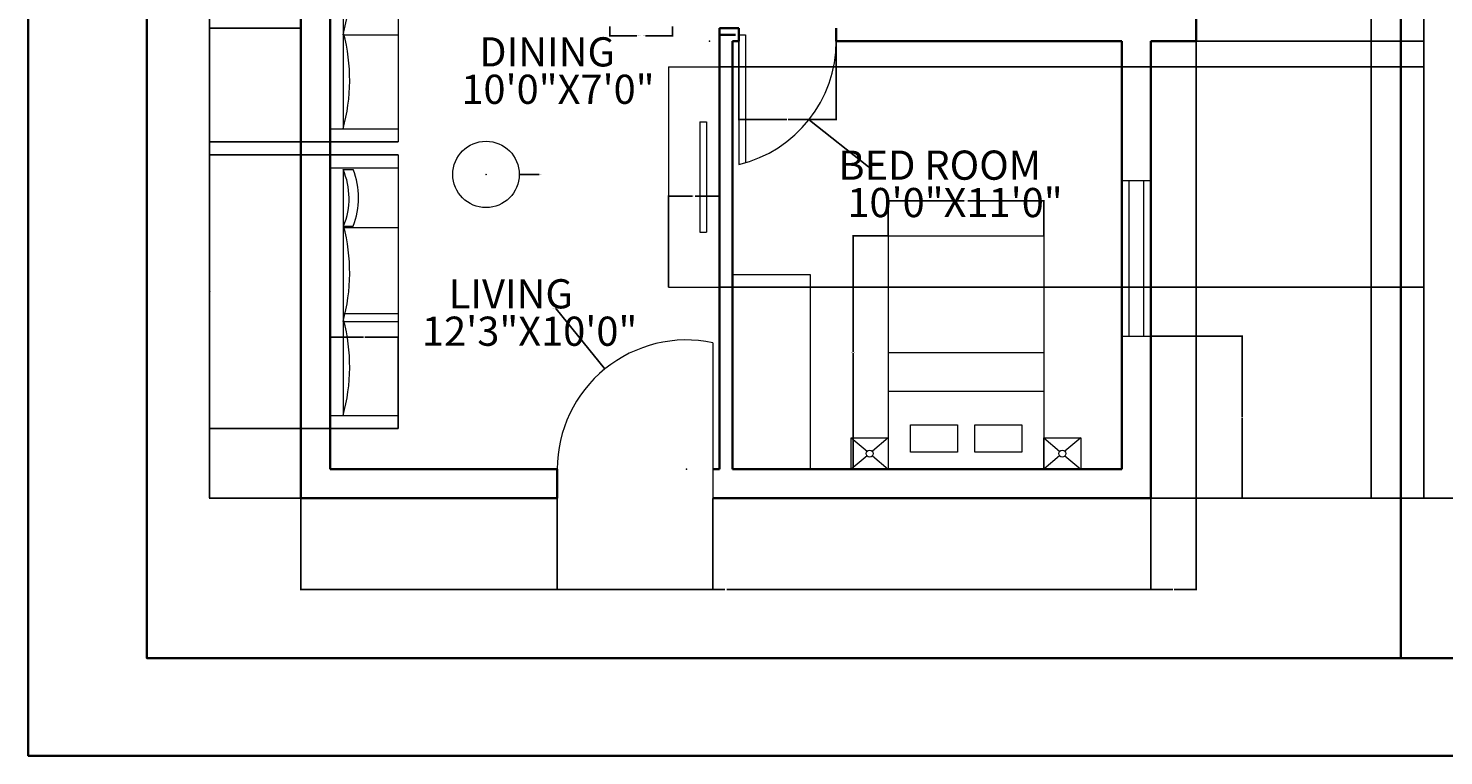
# Model space of a CAD drawing. Units: inches. Extents: x 1762 to 3150, y 1680 to 2382.
# Tile 1 of 6: x 1762 to 2199, y 1680 to 1904. Entities that reach past the tile are written whole.
import ezdxf

# ---------------------------------------------------------------- set-up
doc = ezdxf.new("R2010")
doc.units = ezdxf.units.IN
for name, color, linetype, lineweight in [('A-ANNO-DIMS', 2, 'Continuous', 18), ('A-ANNO-TTLB', 7, 'Continuous', 35), ('A-AREA-IDEN', 7, 'Continuous', 18), ('A-DOOR', 3, 'Continuous', 18), ('A-EQPM', 8, 'Continuous', 18), ('A-GLAZ', 4, 'Continuous', 18), ('A-WALL', 7, 'Continuous', 35)]:
    doc.layers.add(name, color=color, linetype=linetype, lineweight=lineweight)
doc.layers.add('A-FLOR-CASE', color=242, linetype='Continuous', lineweight=18, true_color=0xcd2027)
doc.layers.add('A-FURN', color=51, linetype='Continuous', lineweight=18, true_color=0xf7f281)
doc.styles.get("Standard").update_dxf_attribs({"font": 'arial.ttf'})
doc.dimstyles.get("Standard").update_dxf_attribs({"dimtxt": 0.18, "dimasz": 0.18, "dimexe": 0.18, "dimexo": 0.0625, "dimgap": 0.09, "dimtad": 0, "dimtih": 1, "dimtoh": 1, "dimdec": 4, "dimzin": 0, "dimdsep": 46, "dimtxsty": 'Standard', "dimcen": 0.09, "dimadec": 0, "dimazin": 0, "dimtfac": 1, "dimtdec": 4, "dimtofl": 0, "dimtmove": 0, "dimatfit": 3, "dimfxl": 1, "dimtolj": 1, "dimtzin": 0, "dimarcsym": 0})

# ---------------------------------------------------------------- blocks, each defined once
blk = doc.blocks.new('WINDOW-48IN')
for p, q in [((0, 48), (9, 48)), ((2.25, 48), (2.25, 0)), ((6.75, 48), (6.75, 0)), ((0, 0), (9, 0))]:
    blk.add_line(p, q)
blk = doc.blocks.new('BED-48X72IN')
for p, q in [((0, 72), (48, 72)), ((0, 72), (0, 0)), ((48, 72), (48, 0)), ((0, 36), (48, 36)), ((0, 24), (48, 24))]:
    blk.add_line(p, q)
for points in [[(6.88, 13.68), (21.36, 13.68), (21.36, 5.23), (6.88, 5.23)], [(26.73, 13.68), (41.21, 13.68), (41.21, 5.23), (26.73, 5.23)]]:
    blk.add_lwpolyline(points, close=True)
blk = doc.blocks.new('NIGHTSTAND')
for p, q in [((0, 9.61), (4.85, 5.5)), ((11.36, 9.61), (6.51, 5.5)), ((4.85, 4.1), (0, 0)), ((6.51, 4.1), (11.36, 0))]:
    blk.add_line(p, q)
blk.add_lwpolyline([(0, 9.61), (11.36, 9.61), (11.36, 0), (0, 0)], close=True)
blk.add_circle((5.68, 4.8), 1.08)
blk = doc.blocks.new('*D12')
at = {"layer": 'A-ANNO-DIMS', "color": 0, "lineweight": -2, "transparency": 16777216}
for p, q in [((2027.48, 1839.99), (2016.56, 1839.99)), ((2016.74, 1839.81), (2016.74, 1804.17)), ((2016.74, 1768.17), (2016.74, 1803.81)), ((2027.48, 1767.99), (2016.56, 1767.99))]:
    blk.add_line(p, q, dxfattribs=at)
at = {"layer": 'A-ANNO-DIMS', "color": 0, "transparency": 16777216}
for points in [[(2016.71, 1839.81), (2016.77, 1839.81), (2016.74, 1839.99)], [(2016.71, 1768.17), (2016.77, 1768.17), (2016.74, 1767.99)]]:
    blk.add_solid(points, dxfattribs=at)
at = {"layer": 'Defpoints', "color": 0, "transparency": 16777216}
for p in [(2016.74, 1839.99), (2027.54, 1839.99), (2027.54, 1767.99)]:
    blk.add_point(p, dxfattribs=at)
at = {"layer": 'A-ANNO-DIMS', "color": 0, "transparency": 16777216, "insert": (2016.74, 1803.99), "char_height": 0.18, "attachment_point": 5}
blk.add_mtext('\\A1;BED 72 TYP.', dxfattribs=at)
blk = doc.blocks.new('*D13')
at = {"layer": 'A-ANNO-DIMS', "color": 0, "lineweight": -2, "transparency": 16777216}
for p, q in [((2027.54, 1840.05), (2027.54, 1850.97)), ((2027.72, 1850.79), (2051.01, 1850.79)), ((2075.36, 1850.79), (2052.07, 1850.79)), ((2075.54, 1840.05), (2075.54, 1850.97))]:
    blk.add_line(p, q, dxfattribs=at)
at = {"layer": 'A-ANNO-DIMS', "color": 0, "transparency": 16777216}
for points in [[(2027.72, 1850.82), (2027.72, 1850.76), (2027.54, 1850.79)], [(2075.36, 1850.82), (2075.36, 1850.76), (2075.54, 1850.79)]]:
    blk.add_solid(points, dxfattribs=at)
at = {"layer": 'Defpoints', "color": 0, "transparency": 16777216}
for p in [(2075.54, 1850.79), (2027.54, 1839.99), (2075.54, 1839.99)]:
    blk.add_point(p, dxfattribs=at)
at = {"layer": 'A-ANNO-DIMS', "color": 0, "transparency": 16777216, "insert": (2051.54, 1850.79), "char_height": 0.18, "attachment_point": 5}
blk.add_mtext('\\A1;48 TYP.', dxfattribs=at)
blk = doc.blocks.new('*D22')
at = {"layer": 'A-ANNO-DIMS', "color": 0, "lineweight": -2, "transparency": 16777216}
for p, q in [((1941.79, 1904.51), (1941.79, 1901.5)), ((1961.03, 1904.51), (1961.03, 1901.5)), ((1941.97, 1901.68), (1950.09, 1901.68)), ((1960.85, 1901.68), (1952.73, 1901.68))]:
    blk.add_line(p, q, dxfattribs=at)
at = {"layer": 'A-ANNO-DIMS', "color": 0, "transparency": 16777216}
for points in [[(1941.97, 1901.71), (1941.97, 1901.65), (1941.79, 1901.68)], [(1960.85, 1901.71), (1960.85, 1901.65), (1961.03, 1901.68)]]:
    blk.add_solid(points, dxfattribs=at)
at = {"layer": 'Defpoints', "color": 0, "transparency": 16777216}
for p in [(1941.79, 1904.57), (1961.03, 1904.57), (1941.79, 1901.68)]:
    blk.add_point(p, dxfattribs=at)
at = {"layer": 'A-ANNO-DIMS', "color": 0, "transparency": 16777216, "insert": (1951.41, 1901.68), "char_height": 0.18, "attachment_point": 5}
blk.add_mtext('\\A1;WIDE CHAIR 19 TYP.', dxfattribs=at)
blk = doc.blocks.new('*D33')
at = {"layer": 'A-ANNO-DIMS', "color": 0, "lineweight": -2, "transparency": 16777216}
for p, q in [((1969.475966, 2232.98945), (1818.208466, 2232.98945)), ((1818.388466, 2232.80945), (1818.388466, 1996.16945)), ((1818.388466, 1759.16945), (1818.388466, 1995.80945)), ((1846.475966, 1758.98945), (1818.208466, 1758.98945))]:
    blk.add_line(p, q, dxfattribs=at)
at = {"layer": 'A-ANNO-DIMS', "color": 0, "transparency": 16777216}
for points in [[(1818.358466, 2232.80945), (1818.418466, 2232.80945), (1818.388466, 2232.98945)], [(1818.358466, 1759.16945), (1818.418466, 1759.16945), (1818.388466, 1758.98945)]]:
    blk.add_solid(points, dxfattribs=at)
at = {"layer": 'Defpoints', "color": 0, "transparency": 16777216}
for p in [(1818.388466, 2232.98945), (1969.538466, 2232.98945), (1846.538466, 1758.98945)]:
    blk.add_point(p, dxfattribs=at)
at = {"layer": 'A-ANNO-DIMS', "color": 0, "transparency": 16777216, "insert": (1818.388466, 1995.98945), "char_height": 0.18, "attachment_point": 5}
blk.add_mtext('\\A1;474', dxfattribs=at)
blk = doc.blocks.new('*D35')
at = {"layer": 'A-ANNO-DIMS', "color": 0, "lineweight": -2, "transparency": 16777216}
for p, q in [((2108.6, 1899.99), (2192.87, 1899.99)), ((2192.69, 1899.81), (2192.69, 1829.67)), ((2192.69, 1759.17), (2192.69, 1829.31)), ((2108.6, 1758.99), (2192.87, 1758.99))]:
    blk.add_line(p, q, dxfattribs=at)
at = {"layer": 'A-ANNO-DIMS', "color": 0, "transparency": 16777216}
for points in [[(2192.66, 1899.81), (2192.72, 1899.81), (2192.69, 1899.99)], [(2192.66, 1759.17), (2192.72, 1759.17), (2192.69, 1758.99)]]:
    blk.add_solid(points, dxfattribs=at)
at = {"layer": 'Defpoints', "color": 0, "transparency": 16777216}
for p in [(2108.54, 1899.99), (2192.69, 1899.99), (2108.54, 1758.99)]:
    blk.add_point(p, dxfattribs=at)
at = {"layer": 'A-ANNO-DIMS', "color": 0, "transparency": 16777216, "insert": (2192.69, 1829.49), "char_height": 0.18, "attachment_point": 5}
blk.add_mtext('\\A1;141', dxfattribs=at)
blk = doc.blocks.new('*D36')
at = {"layer": 'A-ANNO-DIMS', "color": 0, "lineweight": -2, "transparency": 16777216}
for p, q in [((2164.6, 1987.99), (2192.87, 1987.99)), ((2192.69, 1987.81), (2192.69, 1944.17)), ((2192.69, 1900.17), (2192.69, 1943.81)), ((2122.6, 1899.99), (2192.87, 1899.99))]:
    blk.add_line(p, q, dxfattribs=at)
at = {"layer": 'A-ANNO-DIMS', "color": 0, "transparency": 16777216}
for points in [[(2192.66, 1987.81), (2192.72, 1987.81), (2192.69, 1987.99)], [(2192.66, 1900.17), (2192.72, 1900.17), (2192.69, 1899.99)]]:
    blk.add_solid(points, dxfattribs=at)
at = {"layer": 'Defpoints', "color": 0, "transparency": 16777216}
for p in [(2164.54, 1987.99), (2192.69, 1987.99), (2122.54, 1899.99)]:
    blk.add_point(p, dxfattribs=at)
at = {"layer": 'A-ANNO-DIMS', "color": 0, "transparency": 16777216, "insert": (2192.69, 1943.99), "char_height": 0.18, "attachment_point": 5}
blk.add_mtext('\\A1;88', dxfattribs=at)
blk = doc.blocks.new('*D39')
at = {"layer": 'A-ANNO-DIMS', "color": 0, "lineweight": -2, "transparency": 16777216}
for p, q in [((1846.54, 1758.93), (1846.54, 1730.66)), ((1925.54, 1758.93), (1925.54, 1730.66)), ((1846.72, 1730.84), (1885.82, 1730.84)), ((1925.36, 1730.84), (1886.26, 1730.84))]:
    blk.add_line(p, q, dxfattribs=at)
at = {"layer": 'A-ANNO-DIMS', "color": 0, "transparency": 16777216}
for points in [[(1846.72, 1730.87), (1846.72, 1730.81), (1846.54, 1730.84)], [(1925.36, 1730.87), (1925.36, 1730.81), (1925.54, 1730.84)]]:
    blk.add_solid(points, dxfattribs=at)
at = {"layer": 'Defpoints', "color": 0, "transparency": 16777216}
for p in [(1846.54, 1758.99), (1925.54, 1758.99), (1925.54, 1730.84)]:
    blk.add_point(p, dxfattribs=at)
at = {"layer": 'A-ANNO-DIMS', "color": 0, "transparency": 16777216, "insert": (1886.04, 1730.84), "char_height": 0.18, "attachment_point": 5}
blk.add_mtext('\\A1;79', dxfattribs=at)
blk = doc.blocks.new('*D40')
at = {"layer": 'A-ANNO-DIMS', "color": 0, "lineweight": -2, "transparency": 16777216}
for p, q in [((1925.54, 1758.93), (1925.54, 1730.66)), ((1973.54, 1758.93), (1973.54, 1730.66)), ((1925.72, 1730.84), (1949.32, 1730.84)), ((1973.36, 1730.84), (1949.76, 1730.84))]:
    blk.add_line(p, q, dxfattribs=at)
at = {"layer": 'A-ANNO-DIMS', "color": 0, "transparency": 16777216}
for points in [[(1925.72, 1730.87), (1925.72, 1730.81), (1925.54, 1730.84)], [(1973.36, 1730.87), (1973.36, 1730.81), (1973.54, 1730.84)]]:
    blk.add_solid(points, dxfattribs=at)
at = {"layer": 'Defpoints', "color": 0, "transparency": 16777216}
for p in [(1925.54, 1758.99), (1973.54, 1758.99), (1973.54, 1730.84)]:
    blk.add_point(p, dxfattribs=at)
at = {"layer": 'A-ANNO-DIMS', "color": 0, "transparency": 16777216, "insert": (1949.54, 1730.84), "char_height": 0.18, "attachment_point": 5}
blk.add_mtext('\\A1;48', dxfattribs=at)
blk = doc.blocks.new('*D41')
at = {"layer": 'A-ANNO-DIMS', "color": 0, "lineweight": -2, "transparency": 16777216}
for p, q in [((1846.54, 1758.93), (1846.54, 1730.66)), ((2108.54, 1758.93), (2108.54, 1730.66)), ((1846.72, 1730.84), (1977.25, 1730.84)), ((2108.36, 1730.84), (1977.83, 1730.84))]:
    blk.add_line(p, q, dxfattribs=at)
at = {"layer": 'A-ANNO-DIMS', "color": 0, "transparency": 16777216}
for points in [[(1846.72, 1730.87), (1846.72, 1730.81), (1846.54, 1730.84)], [(2108.36, 1730.87), (2108.36, 1730.81), (2108.54, 1730.84)]]:
    blk.add_solid(points, dxfattribs=at)
at = {"layer": 'Defpoints', "color": 0, "transparency": 16777216}
for p in [(1846.54, 1758.99), (2108.54, 1758.99), (2108.54, 1730.84)]:
    blk.add_point(p, dxfattribs=at)
at = {"layer": 'A-ANNO-DIMS', "color": 0, "transparency": 16777216, "insert": (1977.54, 1730.84), "char_height": 0.18, "attachment_point": 5}
blk.add_mtext('\\A1;262', dxfattribs=at)
blk = doc.blocks.new('*D42')
at = {"layer": 'A-ANNO-DIMS', "color": 0, "lineweight": -2, "transparency": 16777216}
for p, q in [((2122.54, 1899.93), (2122.54, 1730.66)), ((2108.54, 1758.93), (2108.54, 1730.66)), ((2108.72, 1730.84), (2115.33, 1730.84)), ((2122.36, 1730.84), (2115.75, 1730.84))]:
    blk.add_line(p, q, dxfattribs=at)
at = {"layer": 'A-ANNO-DIMS', "color": 0, "transparency": 16777216}
for points in [[(2108.72, 1730.87), (2108.72, 1730.81), (2108.54, 1730.84)], [(2122.36, 1730.87), (2122.36, 1730.81), (2122.54, 1730.84)]]:
    blk.add_solid(points, dxfattribs=at)
at = {"layer": 'Defpoints', "color": 0, "transparency": 16777216}
for p in [(2122.54, 1899.99), (2108.54, 1758.99), (2122.54, 1730.84)]:
    blk.add_point(p, dxfattribs=at)
at = {"layer": 'A-ANNO-DIMS', "color": 0, "transparency": 16777216, "insert": (2115.54, 1730.84), "char_height": 0.18, "attachment_point": 5}
blk.add_mtext('\\A1;14', dxfattribs=at)
blk = doc.blocks.new('*D47')
at = {"layer": 'A-ANNO-DIMS', "color": 0, "lineweight": -2, "transparency": 16777216}
for p, q in [((1846.48, 1903.99), (1818.21, 1903.99)), ((1818.39, 1903.81), (1818.39, 1831.67)), ((1818.39, 1759.17), (1818.39, 1831.31)), ((1846.48, 1758.99), (1818.21, 1758.99))]:
    blk.add_line(p, q, dxfattribs=at)
at = {"layer": 'A-ANNO-DIMS', "color": 0, "transparency": 16777216}
for points in [[(1818.36, 1903.81), (1818.42, 1903.81), (1818.39, 1903.99)], [(1818.36, 1759.17), (1818.42, 1759.17), (1818.39, 1758.99)]]:
    blk.add_solid(points, dxfattribs=at)
at = {"layer": 'Defpoints', "color": 0, "transparency": 16777216}
for p in [(1818.39, 1903.99), (1846.54, 1903.99), (1846.54, 1758.99)]:
    blk.add_point(p, dxfattribs=at)
at = {"layer": 'A-ANNO-DIMS', "color": 0, "transparency": 16777216, "insert": (1818.39, 1831.49), "char_height": 0.18, "attachment_point": 5}
blk.add_mtext('\\A1;145', dxfattribs=at)
blk = doc.blocks.new('*D48')
at = {"layer": 'A-ANNO-DIMS', "color": 0, "lineweight": -2, "transparency": 16777216}
for p, q in [((2108.6, 1808.99), (2136.87, 1808.99)), ((2136.69, 1808.81), (2136.69, 1784.17)), ((2136.69, 1759.17), (2136.69, 1783.81)), ((2108.6, 1758.99), (2136.87, 1758.99))]:
    blk.add_line(p, q, dxfattribs=at)
at = {"layer": 'A-ANNO-DIMS', "color": 0, "transparency": 16777216}
for points in [[(2136.66, 1808.81), (2136.72, 1808.81), (2136.69, 1808.99)], [(2136.66, 1759.17), (2136.72, 1759.17), (2136.69, 1758.99)]]:
    blk.add_solid(points, dxfattribs=at)
at = {"layer": 'Defpoints', "color": 0, "transparency": 16777216}
for p in [(2108.54, 1808.99), (2108.54, 1758.99), (2136.69, 1758.99)]:
    blk.add_point(p, dxfattribs=at)
at = {"layer": 'A-ANNO-DIMS', "color": 0, "transparency": 16777216, "insert": (2136.69, 1783.99), "char_height": 0.18, "attachment_point": 5}
blk.add_mtext('\\A1;50', dxfattribs=at)
blk = doc.blocks.new('*D51')
at = {"layer": 'A-ANNO-DIMS', "color": 0, "lineweight": -2, "transparency": 16777216}
for p, q in [((1981.54, 1903.93), (1981.54, 1875.66)), ((2011.54, 1903.93), (2011.54, 1875.66)), ((1981.72, 1875.84), (1996.32, 1875.84)), ((2011.36, 1875.84), (1996.76, 1875.84))]:
    blk.add_line(p, q, dxfattribs=at)
at = {"layer": 'A-ANNO-DIMS', "color": 0, "transparency": 16777216}
for points in [[(1981.72, 1875.87), (1981.72, 1875.81), (1981.54, 1875.84)], [(2011.36, 1875.87), (2011.36, 1875.81), (2011.54, 1875.84)]]:
    blk.add_solid(points, dxfattribs=at)
at = {"layer": 'Defpoints', "color": 0, "transparency": 16777216}
for p in [(1981.54, 1903.99), (2011.54, 1903.99), (1981.54, 1875.84)]:
    blk.add_point(p, dxfattribs=at)
at = {"layer": 'A-ANNO-DIMS', "color": 0, "transparency": 16777216, "insert": (1996.54, 1875.84), "char_height": 0.18, "attachment_point": 5}
blk.add_mtext('\\A1;30', dxfattribs=at)
blk = doc.blocks.new('*D56')
at = {"layer": 'A-ANNO-DIMS', "color": 0, "lineweight": -2, "transparency": 16777216}
for p, q in [((2122.6, 1911.99), (2192.87, 1911.99)), ((2192.69, 1911.81), (2192.69, 1906.17)), ((2192.69, 1900.17), (2192.69, 1905.81)), ((2122.6, 1899.99), (2192.87, 1899.99))]:
    blk.add_line(p, q, dxfattribs=at)
at = {"layer": 'A-ANNO-DIMS', "color": 0, "transparency": 16777216}
for points in [[(2192.66, 1911.81), (2192.72, 1911.81), (2192.69, 1911.99)], [(2192.66, 1900.17), (2192.72, 1900.17), (2192.69, 1899.99)]]:
    blk.add_solid(points, dxfattribs=at)
at = {"layer": 'Defpoints', "color": 0, "transparency": 16777216}
for p in [(2122.54, 1911.99), (2192.69, 1911.99), (2122.54, 1899.99)]:
    blk.add_point(p, dxfattribs=at)
at = {"layer": 'A-ANNO-DIMS', "color": 0, "transparency": 16777216, "insert": (2192.69, 1905.99), "char_height": 0.18, "attachment_point": 5}
blk.add_mtext('\\A1;12', dxfattribs=at)
blk = doc.blocks.new('*D59')
at = {"layer": 'A-ANNO-DIMS', "color": 0, "lineweight": -2, "transparency": 16777216}
for p, q in [((1876.48, 1864.99), (1818.21, 1864.99)), ((1818.39, 1864.81), (1818.39, 1822.95)), ((1818.39, 1780.73), (1818.39, 1822.59)), ((1876.48, 1780.55), (1818.21, 1780.55))]:
    blk.add_line(p, q, dxfattribs=at)
at = {"layer": 'A-ANNO-DIMS', "color": 0, "transparency": 16777216}
for points in [[(1818.36, 1864.81), (1818.42, 1864.81), (1818.39, 1864.99)], [(1818.36, 1780.73), (1818.42, 1780.73), (1818.39, 1780.55)]]:
    blk.add_solid(points, dxfattribs=at)
at = {"layer": 'Defpoints', "color": 0, "transparency": 16777216}
for p in [(1818.39, 1864.99), (1876.54, 1864.99), (1876.54, 1780.55)]:
    blk.add_point(p, dxfattribs=at)
at = {"layer": 'A-ANNO-DIMS', "color": 0, "transparency": 16777216, "insert": (1818.39, 1822.77), "char_height": 0.18, "attachment_point": 5}
blk.add_mtext('\\A1;84.44', dxfattribs=at)
blk = doc.blocks.new('*D60')
at = {"layer": 'A-ANNO-DIMS', "color": 0, "lineweight": -2, "transparency": 16777216}
for p, q in [((1876.48, 1963.99), (1818.21, 1963.99)), ((1818.39, 1963.81), (1818.39, 1916.67)), ((1818.39, 1869.17), (1818.39, 1916.31)), ((1876.48, 1868.99), (1818.21, 1868.99))]:
    blk.add_line(p, q, dxfattribs=at)
at = {"layer": 'A-ANNO-DIMS', "color": 0, "transparency": 16777216}
for points in [[(1818.36, 1963.81), (1818.42, 1963.81), (1818.39, 1963.99)], [(1818.36, 1869.17), (1818.42, 1869.17), (1818.39, 1868.99)]]:
    blk.add_solid(points, dxfattribs=at)
at = {"layer": 'Defpoints', "color": 0, "transparency": 16777216}
for p in [(1818.39, 1963.99), (1876.54, 1963.99), (1876.54, 1868.99)]:
    blk.add_point(p, dxfattribs=at)
at = {"layer": 'A-ANNO-DIMS', "color": 0, "transparency": 16777216, "insert": (1818.39, 1916.49), "char_height": 0.18, "attachment_point": 5}
blk.add_mtext('\\A1;95', dxfattribs=at)
blk = doc.blocks.new('*D61')
at = {"layer": 'A-ANNO-DIMS', "color": 0, "lineweight": -2, "transparency": 16777216}
for p, q in [((1855.54, 1780.61), (1855.54, 1808.88)), ((1855.72, 1808.7), (1865.84, 1808.7)), ((1876.36, 1808.7), (1866.24, 1808.7)), ((1876.54, 1780.61), (1876.54, 1808.88))]:
    blk.add_line(p, q, dxfattribs=at)
at = {"layer": 'A-ANNO-DIMS', "color": 0, "transparency": 16777216}
for points in [[(1855.72, 1808.73), (1855.72, 1808.67), (1855.54, 1808.7)], [(1876.36, 1808.73), (1876.36, 1808.67), (1876.54, 1808.7)]]:
    blk.add_solid(points, dxfattribs=at)
at = {"layer": 'Defpoints', "color": 0, "transparency": 16777216}
for p in [(1876.54, 1808.7), (1855.54, 1780.55), (1876.54, 1780.55)]:
    blk.add_point(p, dxfattribs=at)
at = {"layer": 'A-ANNO-DIMS', "color": 0, "transparency": 16777216, "insert": (1866.04, 1808.7), "char_height": 0.18, "attachment_point": 5}
blk.add_mtext('\\A1;21', dxfattribs=at)
blk = doc.blocks.new('*D62')
at = {"layer": 'A-ANNO-DIMS', "color": 0, "lineweight": -2, "transparency": 16777216}
for p, q in [((1975.6, 1892.09), (2192.87, 1892.09)), ((2192.69, 1891.91), (2192.69, 1858.27)), ((2192.69, 1824.27), (2192.69, 1857.91)), ((1975.6, 1824.09), (2192.87, 1824.09))]:
    blk.add_line(p, q, dxfattribs=at)
at = {"layer": 'A-ANNO-DIMS', "color": 0, "transparency": 16777216}
for points in [[(2192.66, 1891.91), (2192.72, 1891.91), (2192.69, 1892.09)], [(2192.66, 1824.27), (2192.72, 1824.27), (2192.69, 1824.09)]]:
    blk.add_solid(points, dxfattribs=at)
at = {"layer": 'Defpoints', "color": 0, "transparency": 16777216}
for p in [(1975.54, 1892.09), (2192.69, 1892.09), (1975.54, 1824.09)]:
    blk.add_point(p, dxfattribs=at)
at = {"layer": 'A-ANNO-DIMS', "color": 0, "transparency": 16777216, "insert": (2192.69, 1858.09), "char_height": 0.18, "attachment_point": 5}
blk.add_mtext('\\A1;68', dxfattribs=at)
blk = doc.blocks.new('*D63')
at = {"layer": 'A-ANNO-DIMS', "color": 0, "lineweight": -2, "transparency": 16777216}
for p, q in [((1959.8, 1824.15), (1959.8, 1852.42)), ((1959.98, 1852.24), (1967.28, 1852.24)), ((1975.36, 1852.24), (1968.05, 1852.24)), ((1975.54, 1824.15), (1975.54, 1852.42))]:
    blk.add_line(p, q, dxfattribs=at)
at = {"layer": 'A-ANNO-DIMS', "color": 0, "transparency": 16777216}
for points in [[(1959.98, 1852.27), (1959.98, 1852.21), (1959.8, 1852.24)], [(1975.36, 1852.27), (1975.36, 1852.21), (1975.54, 1852.24)]]:
    blk.add_solid(points, dxfattribs=at)
at = {"layer": 'Defpoints', "color": 0, "transparency": 16777216}
for p in [(1975.54, 1852.24), (1959.8, 1824.09), (1975.54, 1824.09)]:
    blk.add_point(p, dxfattribs=at)
at = {"layer": 'A-ANNO-DIMS', "color": 0, "transparency": 16777216, "insert": (1967.67, 1852.24), "char_height": 0.18, "attachment_point": 5}
blk.add_mtext('\\A1;15.74', dxfattribs=at)
blk = doc.blocks.new('*D65')
at = {"layer": 'A-ANNO-DIMS', "color": 0, "lineweight": -2, "transparency": 16777216}
for p, q in [((2364.876105, 2232.98945), (2176.268936, 2232.98945)), ((2176.448936, 2232.80945), (2176.448936, 1996.16945)), ((2176.448936, 1759.16945), (2176.448936, 1995.80945)), ((2239.876105, 1758.98945), (2176.268936, 1758.98945))]:
    blk.add_line(p, q, dxfattribs=at)
at = {"layer": 'A-ANNO-DIMS', "color": 0, "transparency": 16777216}
for points in [[(2176.418936, 2232.80945), (2176.478936, 2232.80945), (2176.448936, 2232.98945)], [(2176.418936, 1759.16945), (2176.478936, 1759.16945), (2176.448936, 1758.98945)]]:
    blk.add_solid(points, dxfattribs=at)
at = {"layer": 'Defpoints', "color": 0, "transparency": 16777216}
for p in [(2176.448936, 2232.98945), (2364.938605, 2232.98945), (2239.938605, 1758.98945)]:
    blk.add_point(p, dxfattribs=at)
at = {"layer": 'A-ANNO-DIMS', "color": 0, "transparency": 16777216, "insert": (2176.448936, 1995.98945), "char_height": 0.18, "attachment_point": 5}
blk.add_mtext('\\A1;474', dxfattribs=at)
blk = doc.blocks.new('*D97')
at = {"layer": 'A-ANNO-DIMS', "color": 0, "lineweight": -2, "transparency": 16777216}
for p, q in [((1925, 1817.47), (1925.18, 1817.47)), ((1925.18, 1817.47), (1940.14, 1799.05)), ((1965.29, 1767.99), (1965.47, 1767.99)), ((1965.38, 1767.9), (1965.38, 1768.08))]:
    blk.add_line(p, q, dxfattribs=at)
at = {"layer": 'A-ANNO-DIMS', "color": 0, "transparency": 16777216}
blk.add_solid([(1940.17, 1799.07), (1940.12, 1799.03), (1940.26, 1798.91)], dxfattribs=at)
at = {"layer": 'Defpoints', "color": 0, "transparency": 16777216}
for p in [(1940.26, 1798.91), (1965.38, 1767.99)]:
    blk.add_point(p, dxfattribs=at)
at = {"layer": 'A-ANNO-DIMS', "color": 0, "transparency": 16777216, "insert": (1924.52, 1817.47), "char_height": 0.18, "attachment_point": 5}
blk.add_mtext('\\A1;R39.84', dxfattribs=at)
blk = doc.blocks.new('*D98')
at = {"layer": 'A-ANNO-DIMS', "color": 0, "lineweight": -2, "transparency": 16777216}
for p, q in [((1972.38, 1899.99), (1972.56, 1899.99)), ((1972.47, 1899.9), (1972.47, 1900.08)), ((2021.53, 1861.26), (2003.28, 1875.67)), ((2021.71, 1861.26), (2021.53, 1861.26))]:
    blk.add_line(p, q, dxfattribs=at)
at = {"layer": 'A-ANNO-DIMS', "color": 0, "transparency": 16777216}
blk.add_solid([(2003.29, 1875.69), (2003.26, 1875.65), (2003.13, 1875.78)], dxfattribs=at)
at = {"layer": 'Defpoints', "color": 0, "transparency": 16777216}
for p in [(1972.47, 1899.99), (2003.13, 1875.78)]:
    blk.add_point(p, dxfattribs=at)
at = {"layer": 'A-ANNO-DIMS', "color": 0, "transparency": 16777216, "insert": (2022.19, 1861.26), "char_height": 0.18, "attachment_point": 5}
blk.add_mtext('\\A1;R39.07', dxfattribs=at)
blk = doc.blocks.new('*D102')
at = {"layer": 'A-ANNO-DIMS', "color": 0, "lineweight": -2, "transparency": 16777216}
for p, q in [((1903.5, 1858.9), (1903.68, 1858.9)), ((1903.59, 1858.81), (1903.59, 1858.99)), ((1919.99, 1858.9), (1914.02, 1858.9))]:
    blk.add_line(p, q, dxfattribs=at)
at = {"layer": 'A-ANNO-DIMS', "color": 0, "transparency": 16777216}
blk.add_solid([(1914.02, 1858.93), (1914.02, 1858.87), (1913.84, 1858.9)], dxfattribs=at)
at = {"layer": 'Defpoints', "color": 0, "transparency": 16777216}
for p in [(1893.34, 1858.9), (1913.84, 1858.9)]:
    blk.add_point(p, dxfattribs=at)
at = {"layer": 'A-ANNO-DIMS', "color": 0, "transparency": 16777216, "insert": (1920.41, 1858.9), "char_height": 0.18, "attachment_point": 5}
blk.add_mtext('\\A1;∅20.5', dxfattribs=at)

msp = doc.modelspace()

# ---------------------------------------------------------------- linework, layer by layer
at = {"layer": 'A-ANNO-TTLB'}
msp.add_line((2185.5413, 2359.5805), (2185.5413, 1709.6712), dxfattribs=at)
for points in [[(1762.4998, 2382.3025), (3150.3176, 2382.3025), (3150.3176, 1679.5742), (1762.4998, 1679.5742)], [(1799.0337, 2359.5805), (3111.4319, 2359.5805), (3111.4319, 1709.6712), (1799.0337, 1709.6712)]]:
    msp.add_lwpolyline(points, close=True, dxfattribs=at)
at = {"layer": 'A-DOOR'}
for p, q in [((1981.5385, 1901.9895), (1983.5385, 1901.9895)), ((1981.5385, 1899.9895), (1981.5385, 1861.9895)), ((1983.5385, 1901.9895), (1983.5385, 1862.523)), ((1973.5385, 1806.9895), (1973.5385, 1758.9895))]:
    msp.add_line(p, q, dxfattribs=at)
for centre, radius, start, end in [((1972.4718, 1899.9895), 39.0667, 283.419674, 360), ((1965.3822, 1767.9894), 39.8438, 78.187718, 180)]:
    msp.add_arc(centre, radius, start, end, dxfattribs=at)
at = {"layer": 'A-EQPM'}
for p, q in [((1969.5385, 1875.0876), (1969.5385, 1841.0876)), ((1969.5385, 1875.0876), (1971.5385, 1875.0876)), ((1971.5385, 1875.0876), (1971.5385, 1841.0876)), ((1969.5385, 1841.0876), (1971.5385, 1841.0876))]:
    msp.add_line(p, q, dxfattribs=at)
at = {"layer": 'A-FLOR-CASE'}
for p, q in [((1979.5385, 1827.9895), (2003.5385, 1827.9895)), ((2003.5385, 1827.9895), (2003.5385, 1767.9894))]:
    msp.add_line(p, q, dxfattribs=at)
at = {"layer": 'A-FURN'}
for p, q in [((1876.5385, 1963.9895), (1876.5385, 1868.9895)), ((1859.5385, 1959.375), (1859.5385, 1872.9895)), ((1859.5385, 1948.868), (1859.5385, 1872.9895)), ((1859.5385, 1901.9895), (1876.5385, 1901.9895)), ((1959.7976, 1892.0876), (1959.7976, 1824.0876)), ((1959.7976, 1892.0876), (1975.5385, 1892.0876)), ((1855.5385, 1872.9895), (1876.5385, 1872.9895)), ((1855.5385, 1868.9895), (1876.5385, 1868.9895)), ((1855.5385, 1868.9895), (1876.5385, 1868.9895)), ((1855.5385, 1864.9895), (1876.5385, 1864.9895)), ((1855.5385, 1864.9895), (1876.5385, 1864.9895)), ((1876.5385, 1864.9895), (1876.5385, 1780.5457)), ((1855.5385, 1860.9895), (1876.5385, 1860.9895)), ((1859.5385, 1860.4242), (1859.5385, 1784.5457)), ((1859.5385, 1860.4242), (1862.6768, 1860.4242)), ((1859.5385, 1842.5457), (1876.5385, 1842.5457)), ((1859.7077, 1842.9652), (1862.6201, 1842.9652)), ((1959.7976, 1824.0876), (1975.5385, 1824.0876)), ((1859.5385, 1815.9895), (1876.5385, 1815.9895)), ((1859.5385, 1813.5457), (1876.5385, 1813.5457)), ((1855.5385, 1784.5457), (1876.5385, 1784.5457)), ((1855.5385, 1780.5457), (1876.5385, 1780.5457))]:
    msp.add_line(p, q, dxfattribs=at)
msp.add_circle((1903.5902, 1858.9023), 10.2492, dxfattribs=at)
for centre, radius, start, end in [((1804.8495, 1917.0143), 56.7154, 344.638036, 14.70288), ((1804.8495, 1888.0143), 56.7154, 344.638036, 14.70288), ((1838.7215, 1851.4921), 22.6523, 337.887546, 23.223033), ((1840.191, 1851.7676), 24.0946, 338.572403, 21.055804), ((1804.8495, 1828.5705), 56.7154, 344.638036, 14.70288), ((1804.8495, 1799.5705), 56.7154, 344.638036, 14.70288)]:
    msp.add_arc(centre, radius, start, end, dxfattribs=at)
at = {"layer": 'A-WALL'}
for p, q in [((1846.5385, 2120.9895), (1846.5385, 1758.9895)), ((2122.5385, 1987.9895), (2122.5385, 1899.9895)), ((1855.5385, 1975.9895), (1855.5385, 1767.9894)), ((1975.5385, 1903.9895), (1975.5385, 1767.9894)), ((1981.5385, 1903.9895), (1975.5385, 1903.9895)), ((1981.5385, 1903.9895), (1981.5385, 1899.9895)), ((2011.5385, 1903.9895), (2011.5385, 1899.9895)), ((1975.5385, 1901.9895), (1980.5385, 1901.9895)), ((1979.5385, 1899.9895), (1979.5385, 1767.9894)), ((1979.5385, 1899.9895), (1981.5385, 1899.9895)), ((2011.5385, 1899.9895), (2099.5385, 1899.9895)), ((2099.5385, 1899.9895), (2099.5385, 1767.9894)), ((2108.5385, 1899.9895), (2108.5385, 1758.9895)), ((2108.5385, 1899.9895), (2122.5385, 1899.9895)), ((1855.5385, 1767.9894), (1925.5385, 1767.9894)), ((1925.5385, 1767.9894), (1925.5385, 1758.9895)), ((1973.5385, 1767.9894), (1975.5385, 1767.9894)), ((1979.5385, 1767.9894), (2099.5385, 1767.9894)), ((1846.5385, 1758.9895), (1925.5385, 1758.9895)), ((1973.5385, 1758.9895), (2108.5385, 1758.9895))]:
    msp.add_line(p, q, dxfattribs=at)

# ---------------------------------------------------------------- block references
at = {"layer": 'A-FURN'}
for name, p in [('BED-48X72IN', (2027.538, 1767.989)), ('NIGHTSTAND', (2016.181, 1767.989)), ('NIGHTSTAND', (2075.5382, 1767.989))]:
    msp.add_blockref(name, p, dxfattribs=at)
at = {"layer": 'A-GLAZ'}
msp.add_blockref('WINDOW-48IN', (2099.538, 1808.989), dxfattribs=at)

# ---------------------------------------------------------------- texts
at = {"layer": 'A-AREA-IDEN'}
for s, p in [('    DINING', (1890.4796, 1892.2119)), ('  10\'0"X7\'0"', (1890.4796, 1880.6728)), ('BED ROOM', (2012.2186, 1857.2645)), (' 10\'0"X11\'0"', (2012.2186, 1845.7254)), ('    LIVING ', (1881.0978, 1817.5729)), (' 12\'3"X10\'0"', (1881.0978, 1806.0338))]:
    msp.add_text(s, height=9, dxfattribs=at).set_placement(p)

# ---------------------------------------------------------------- dimensions: what is measured, and where the dimension line sits
at = {"layer": 'A-ANNO-DIMS'}
for base, p1, p2, angle, override, picture, middle in [((1818.3885, 2232.9895), (1846.5385, 1758.9895), (1969.5385, 2232.9895), 90, {"dimdec": 0, "dimlfac": 1, "dimrnd": 0, "dimzin": 0, "dimdsep": 46, "dimlunit": 2}, '*D33', (1818.3885, 1995.9895)), ((2176.4489, 2232.9895), (2239.9386, 1758.9895), (2364.9386, 2232.9895), 90, {"dimdec": 0, "dimlfac": 1, "dimrnd": 0, "dimzin": 0, "dimdsep": 46, "dimlunit": 2}, '*D65', (2176.4489, 1995.9894)), ((2192.6885, 1987.9895), (2122.5385, 1899.9895), (2164.5385, 1987.9895), 90, {"dimdec": 0, "dimlfac": 1, "dimrnd": 0, "dimzin": 0, "dimdsep": 46, "dimlunit": 2}, '*D36', (2192.6885, 1943.9895)), ((1818.3885, 1963.9895), (1876.5385, 1868.9895), (1876.5385, 1963.9895), 90, {"dimdec": 0, "dimlfac": 1, "dimrnd": 0, "dimzin": 0, "dimdsep": 46, "dimlunit": 2}, '*D60', (1818.3885, 1916.4895)), ((2192.6885, 1911.9895), (2122.5385, 1899.9895), (2122.5385, 1911.9895), 90, {"dimdec": 0, "dimlfac": 1, "dimrnd": 0, "dimzin": 0, "dimdsep": 46, "dimlunit": 2}, '*D56', (2192.6885, 1905.9895)), ((1818.3885, 1903.9895), (1846.5385, 1758.9895), (1846.5385, 1903.9895), 90, {"dimdec": 0, "dimlfac": 1, "dimrnd": 0, "dimzin": 0, "dimdsep": 46, "dimlunit": 2}, '*D47', (1818.3885, 1831.4895)), ((1981.5385, 1875.8394), (2011.5385, 1903.9895), (1981.5385, 1903.9895), 180, {"dimdec": 0, "dimlfac": 1, "dimrnd": 0, "dimzin": 0, "dimdsep": 46, "dimlunit": 2}, '*D51', (1996.5385, 1875.8394)), ((2192.6885, 1899.9895), (2108.5385, 1758.9895), (2108.5385, 1899.9895), 90, {"dimdec": 0, "dimlfac": 1, "dimrnd": 0, "dimzin": 0, "dimdsep": 46, "dimlunit": 2}, '*D35', (2192.6885, 1829.4895)), ((2192.6885, 1892.0876), (1975.5385, 1824.0876), (1975.5385, 1892.0876), 90, {"dimdec": 0, "dimlfac": 1, "dimrnd": 0, "dimzin": 0, "dimdsep": 46, "dimlunit": 2}, '*D62', (2192.6885, 1858.0876)), ((1818.3885, 1864.9895), (1876.5385, 1780.5457), (1876.5385, 1864.9895), 90, {"dimdec": 2, "dimlfac": 1, "dimrnd": 0, "dimzin": 0, "dimdsep": 46, "dimlunit": 2}, '*D59', (1818.3885, 1822.7676)), ((2136.6885, 1758.9895), (2108.5385, 1808.9895), (2108.5385, 1758.9895), 270, {"dimdec": 0, "dimlfac": 1, "dimrnd": 0, "dimzin": 0, "dimdsep": 46, "dimlunit": 2}, '*D48', (2136.6885, 1783.9895))]:
    dim = msp.add_linear_dim(base=base, p1=p1, p2=p2, angle=angle, dimstyle='Standard', override=override, dxfattribs=at)
    dim.commit()
    dim.dimension.update_dxf_attribs({"geometry": picture, "text_midpoint": middle})
for base, p1, p2, angle, text, picture, middle in [((1941.793, 1901.6842), (1961.0299, 1904.5697), (1941.793, 1904.5697), 180, 'WIDE CHAIR <> TYP.', '*D22', (1951.4115, 1901.6842)), ((2016.7385, 1839.9895), (2027.5385, 1767.9894), (2027.5385, 1839.9895), 90, 'BED <> TYP.', '*D12', (2016.7385, 1803.9895))]:
    dim = msp.add_linear_dim(base=base, p1=p1, p2=p2, angle=angle, text=text, dimstyle='Standard', override={"dimdec": 0, "dimlfac": 1, "dimrnd": 0, "dimzin": 0, "dimdsep": 46, "dimlunit": 2}, dxfattribs=at)
    dim.commit()
    dim.dimension.update_dxf_attribs({"geometry": picture, "text_midpoint": middle})
for center, mpoint, picture, middle in [((1972.4718, 1899.9895), (2003.1347, 1875.7822), '*D98', (2022.1923, 1861.2579)), ((1965.3822, 1767.9894), (1940.2571, 1798.9128), '*D97', (1924.5226, 1817.4668))]:
    dim = msp.add_radius_dim(center=center, mpoint=mpoint, dimstyle='Standard', override={"dimdec": 2, "dimlfac": 1, "dimrnd": 0, "dimzin": 0, "dimdsep": 46, "dimlunit": 2}, dxfattribs=at)
    dim.commit()
    dim.dimension.update_dxf_attribs({"geometry": picture, "text_midpoint": middle, "dimtype": 164})
for base, p1, p2, override, picture, middle in [((2122.5385, 1730.8394), (2108.5385, 1758.9895), (2122.5385, 1899.9895), {"dimdec": 0, "dimlfac": 1, "dimrnd": 0, "dimzin": 0, "dimdsep": 46, "dimlunit": 2}, '*D42', (2115.5385, 1730.8394)), ((1975.5385, 1852.2376), (1959.7976, 1824.0876), (1975.5385, 1824.0876), {"dimdec": 2, "dimlfac": 1, "dimrnd": 0, "dimzin": 0, "dimdsep": 46, "dimlunit": 2}, '*D63', (1967.668, 1852.2376)), ((1876.5385, 1808.6957), (1855.5385, 1780.5457), (1876.5385, 1780.5457), {"dimdec": 0, "dimlfac": 1, "dimrnd": 0, "dimzin": 0, "dimdsep": 46, "dimlunit": 2}, '*D61', (1866.0385, 1808.6957)), ((1925.5385, 1730.8394), (1846.5385, 1758.9895), (1925.5385, 1758.9895), {"dimdec": 0, "dimlfac": 1, "dimrnd": 0, "dimzin": 0, "dimdsep": 46, "dimlunit": 2}, '*D39', (1886.0385, 1730.8394)), ((2108.5385, 1730.8394), (1846.5385, 1758.9895), (2108.5385, 1758.9895), {"dimdec": 0, "dimlfac": 1, "dimrnd": 0, "dimzin": 0, "dimdsep": 46, "dimlunit": 2}, '*D41', (1977.5385, 1730.8394)), ((1973.5385, 1730.8394), (1925.5385, 1758.9895), (1973.5385, 1758.9895), {"dimdec": 0, "dimlfac": 1, "dimrnd": 0, "dimzin": 0, "dimdsep": 46, "dimlunit": 2}, '*D40', (1949.5385, 1730.8394))]:
    dim = msp.add_linear_dim(base=base, p1=p1, p2=p2, dimstyle='Standard', override=override, dxfattribs=at)
    dim.commit()
    dim.dimension.update_dxf_attribs({"geometry": picture, "text_midpoint": middle})
dim = msp.add_diameter_dim_2p(p1=(1893.341, 1858.9025), p2=(1913.8394, 1858.902), dimstyle='Standard', override={"dimdec": 1, "dimlfac": 1, "dimrnd": 0, "dimzin": 0, "dimdsep": 46, "dimlunit": 2}, dxfattribs=at)
dim.commit()
dim.dimension.update_dxf_attribs({"geometry": '*D102', "text_midpoint": (1919.989, 1858.9018), "dimtype": 163})
dim = msp.add_linear_dim(base=(2075.5385, 1850.7895), p1=(2027.5385, 1839.9895), p2=(2075.5385, 1839.9895), text='<> TYP.', dimstyle='Standard', override={"dimdec": 0, "dimlfac": 1, "dimrnd": 0, "dimzin": 0, "dimdsep": 46, "dimlunit": 2}, dxfattribs=at)
dim.commit()
dim.dimension.update_dxf_attribs({"geometry": '*D13', "text_midpoint": (2051.5385, 1850.7895)})

doc.saveas('drawing.dxf')
